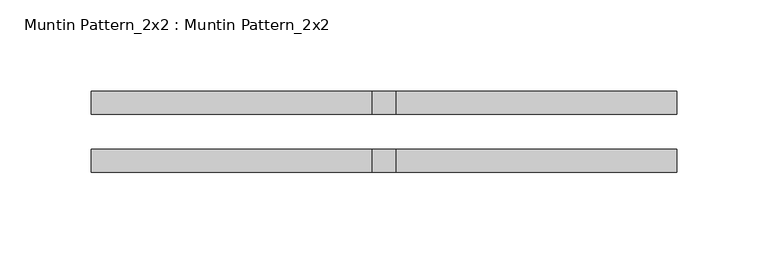
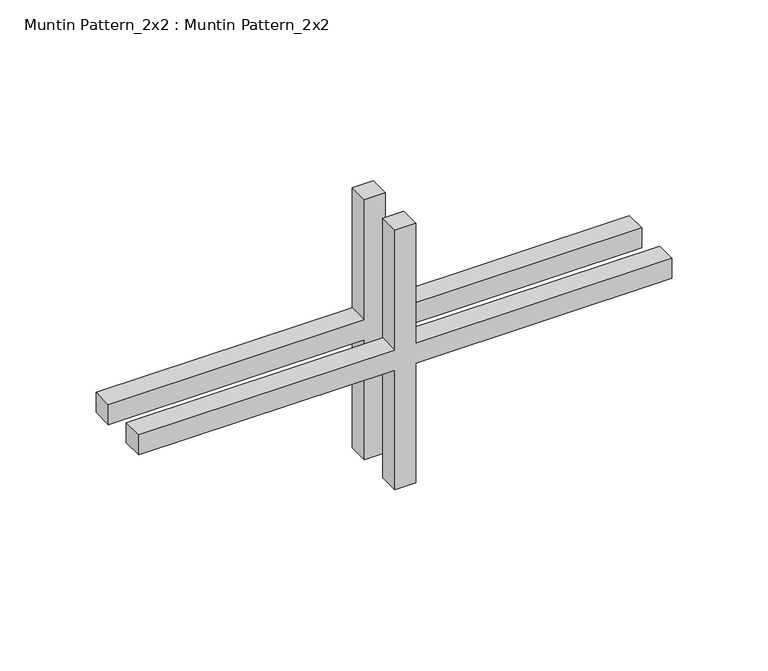
"""IFC4 building model written with IfcOpenShell, lengths in millimetres: proxy geometry, Muntin Pattern_2x2 : Muntin Pattern_2x2."""

from ifc_helpers import new_model, si_unit, frame, origin, place, context, project, spatial, polyline, outline, extrude, source, transform, mapped, element, save


def muntin_pattern_2x2_muntin_pattern_2x2_604ffb00(model_context):
    return source(origin(), model_context, "Body", "SweptSolid", [
        extrude(outline(polyline([(88.9, -6.35), (88.9, -160.3375), (76.2, -160.3375), (76.2, -6.35), (0.0, -6.35), (0.0, 6.35), (76.2, 6.35), (76.2, 160.3375), (88.9, 160.3375), (88.9, 6.35), (165.1, 6.35), (165.1, -6.35), (88.9, -6.35)])), frame((0.0, -22.225, 0.0), z_axis=(0.0, 1.0, 0.0), x_axis=(0.0, 0.0, 1.0)), (0.0, 0.0, 1.0), 12.7),
        extrude(outline(polyline([(88.9, -6.35), (88.9, -160.3375), (76.2, -160.3375), (76.2, -6.35), (0.0, -6.35), (0.0, 6.35), (76.2, 6.35), (76.2, 160.3375), (88.9, 160.3375), (88.9, 6.35), (165.1, 6.35), (165.1, -6.35), (88.9, -6.35)])), frame((0.0, 9.525, 0.0), z_axis=(0.0, 1.0, 0.0), x_axis=(0.0, 0.0, 1.0)), (0.0, 0.0, 1.0), 12.7),
    ])


if __name__ == "__main__":
    model = new_model("IFC4")
    model_context = context("Model", 3, world=origin())
    ifc_project = project(units=[si_unit("LENGTHUNIT", "METRE", prefix="MILLI")], contexts=[model_context])
    site = spatial("IfcSite", under=ifc_project)
    building = spatial("IfcBuilding", under=site)
    placement = place(None, origin())
    muntin_pattern_2x2_muntin_pattern_2x2_shape = muntin_pattern_2x2_muntin_pattern_2x2_604ffb00(model_context)
    element("IfcBuildingElementProxy", 1, Name="Muntin Pattern_2x2 : Muntin Pattern_2x2", ObjectType="Muntin Pattern_2x2 : Muntin Pattern_2x2", at=placement, inside=building, context=model_context, shape_type="MappedRepresentation", body=[
        mapped(muntin_pattern_2x2_muntin_pattern_2x2_shape, transform((0.0, 0.0, 0.0), x_axis=(1.0, 0.0, 0.0), y_axis=(0.0, 1.0, 0.0), z_axis=(0.0, 0.0, 1.0))),
    ])
    save(model, "model.ifc")

# Revit data of these elements
# Type "Muntin Pattern_2x2 : Muntin Pattern_2x2"
#   Width [instance default] = 4' - 0"
#   Thickness = 0' - 0 1/2"
#   Height [instance default] = 4' - 0"
#   Distance = 0' - 0 3/4"
#   Interior Material [instance default] = none
#   Exterior Material [instance default] = none
#   Default Elevation = 0
# Element 1 (IfcBuildingElementProxy, "Muntin Pattern_2x2 : Muntin Pattern_2x2")
#   Width = 1' - 0 5/8"
#   Height = 0' - 6 1/2"
#   Interior Material = Wood - Stained
#   Exterior Material = Clad - White
#   Materials on its faces: "Clad - White", "Wood - Stained"
# Materials
#   "Clad - White": class "Wood", colour RGB 242 242 238, transparency 0, Cost = 0
#   "Wood - Stained": class "Wood", colour RGB 224 178 126, transparency 0, Cost = 0
